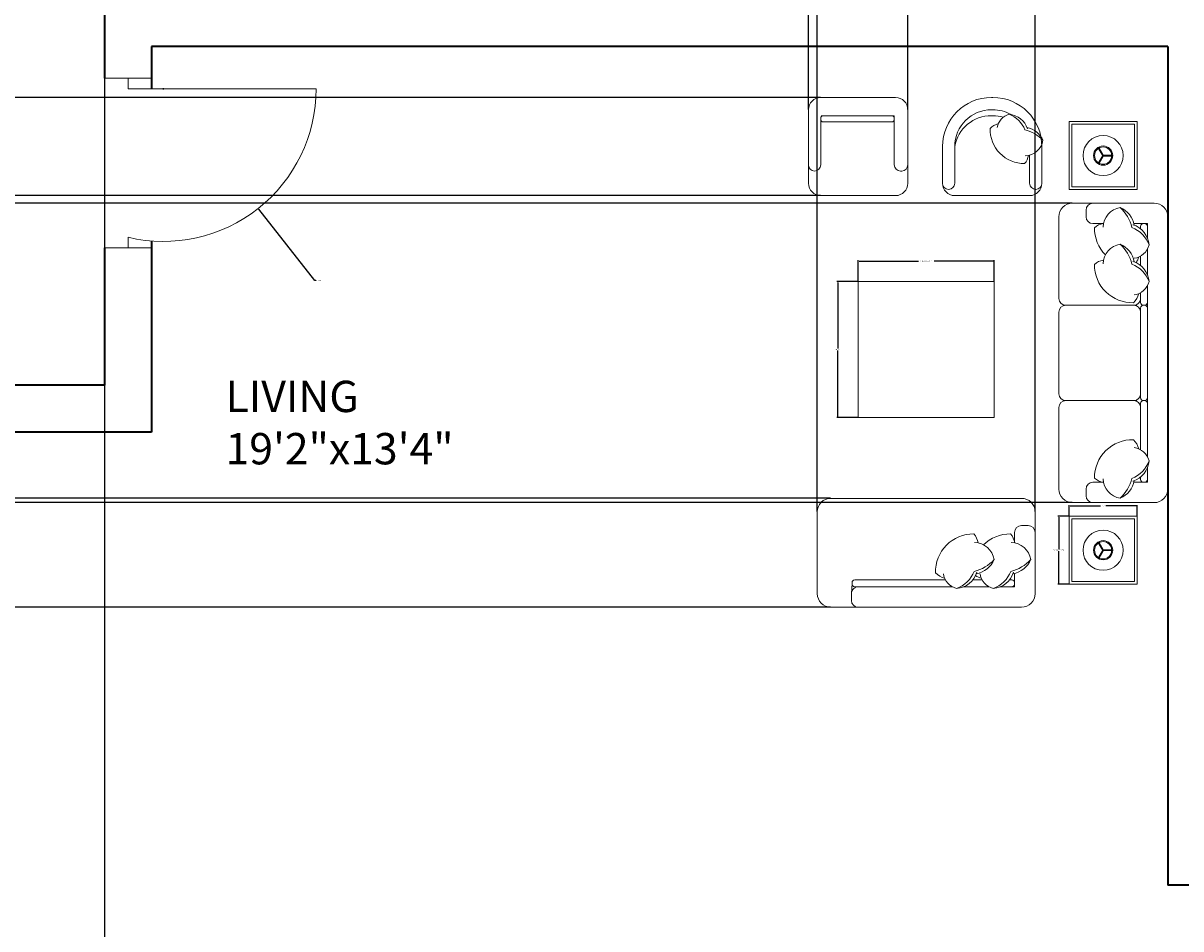
# Model space of a CAD drawing. Units: inches. Extents: x 1902 to 2626, y 1199 to 2408.
# Tile 4 of 9: x 2113 to 2334, y 1644 to 1817. Entities that reach past the tile are written whole.
import ezdxf

# ---------------------------------------------------------------- set-up
doc = ezdxf.new("R2010")
doc.units = ezdxf.units.IN
for name, color, linetype, lineweight in [('A-ANNO-DIMS', 2, 'Continuous', 18), ('A-AREA-IDEN', 7, 'Continuous', 18), ('A-DOOR', 31, 'Continuous', 18), ('A-FURN', 8, 'Continuous', 13), ('A-WALL', 7, 'Continuous', 35)]:
    doc.layers.add(name, color=color, linetype=linetype, lineweight=lineweight)
doc.styles.get("Standard").update_dxf_attribs({"font": 'arial.ttf'})
doc.dimstyles.get("Standard").update_dxf_attribs({"dimtxt": 0.18, "dimasz": 0.18, "dimexe": 0.18, "dimexo": 0.0625, "dimgap": 0.09, "dimtad": 0, "dimtih": 1, "dimtoh": 1, "dimdec": 4, "dimzin": 0, "dimdsep": 46, "dimtxsty": 'Standard', "dimcen": 0.09, "dimadec": 0, "dimazin": 0, "dimtfac": 1, "dimtdec": 4, "dimtofl": 0, "dimtmove": 0, "dimatfit": 3, "dimfxl": 1, "dimtolj": 1, "dimtzin": 0, "dimarcsym": 0})

# ---------------------------------------------------------------- blocks, each defined once
blk = doc.blocks.new('TABLE-END-WITH-LAMP')
for p, q in [((6.45, 6.47), (5.53, 8.06)), ((6.59, 6.55), (5.67, 8.14)), ((6.45, 6.55), (5.53, 4.96)), ((6.59, 6.47), (5.67, 4.88)), ((6.52, 6.59), (8.35, 6.59)), ((6.52, 6.43), (8.35, 6.43))]:
    blk.add_line(p, q)
at = {"ltscale": 0.03}
blk.add_lwpolyline([(0.01, 0), (0.01, 13.02), (13.03, 13.02), (13.03, 0)], close=True, dxfattribs=at)
blk.add_lwpolyline([(0.53, 12.5), (0.53, 0.52), (12.51, 0.52), (12.51, 12.5)], close=True)
for radius in [3.84, 1.84, 1.65]:
    blk.add_circle((6.52, 6.51), radius)
blk = doc.blocks.new('TABLE-COFFEE-SQUARE')
at = {"ltscale": 0.03}
blk.add_lwpolyline([(0, 26.05), (0, 0), (26.05, 0), (26.05, 26.05)], close=True, dxfattribs=at)
blk = doc.blocks.new('*D24')
at = {"layer": 'A-ANNO-DIMS', "color": 0, "lineweight": -2, "transparency": 16777216}
for p, q in [((2312.9, 1722.59), (2310.83, 1722.59)), ((2311.01, 1722.41), (2311.01, 1716.26)), ((2311.01, 1709.75), (2311.01, 1715.9)), ((2312.9, 1709.57), (2310.83, 1709.57))]:
    blk.add_line(p, q, dxfattribs=at)
at = {"layer": 'A-ANNO-DIMS', "color": 0, "transparency": 16777216}
for points in [[(2310.98, 1722.41), (2311.04, 1722.41), (2311.01, 1722.59)], [(2310.98, 1709.75), (2311.04, 1709.75), (2311.01, 1709.57)]]:
    blk.add_solid(points, dxfattribs=at)
at = {"layer": 'Defpoints', "color": 0, "transparency": 16777216}
for p in [(2311.01, 1722.59), (2312.97, 1722.59), (2312.97, 1709.57)]:
    blk.add_point(p, dxfattribs=at)
at = {"layer": 'A-ANNO-DIMS', "color": 0, "transparency": 16777216, "insert": (2311.01, 1716.08), "char_height": 0.18, "attachment_point": 5}
blk.add_mtext('\\A1;END TABLE 13 TYP.', dxfattribs=at)
blk = doc.blocks.new('*D25')
at = {"layer": 'A-ANNO-DIMS', "color": 0, "lineweight": -2, "transparency": 16777216}
for p, q in [((2312.97, 1722.66), (2312.97, 1724.73)), ((2313.15, 1724.55), (2318.96, 1724.55)), ((2325.81, 1724.55), (2320, 1724.55)), ((2325.99, 1722.66), (2325.99, 1724.73))]:
    blk.add_line(p, q, dxfattribs=at)
at = {"layer": 'A-ANNO-DIMS', "color": 0, "transparency": 16777216}
for points in [[(2313.15, 1724.58), (2313.15, 1724.52), (2312.97, 1724.55)], [(2325.81, 1724.58), (2325.81, 1724.52), (2325.99, 1724.55)]]:
    blk.add_solid(points, dxfattribs=at)
at = {"layer": 'Defpoints', "color": 0, "transparency": 16777216}
for p in [(2325.99, 1724.55), (2312.97, 1722.59), (2325.99, 1722.59)]:
    blk.add_point(p, dxfattribs=at)
at = {"layer": 'A-ANNO-DIMS', "color": 0, "transparency": 16777216, "insert": (2319.48, 1724.55), "char_height": 0.18, "attachment_point": 5}
blk.add_mtext('\\A1;13 TYP.', dxfattribs=at)
blk = doc.blocks.new('*D26')
at = {"layer": 'A-ANNO-DIMS', "color": 0, "lineweight": -2, "transparency": 16777216}
for p, q in [((2272.59, 1767.59), (2272.59, 1771.62)), ((2272.77, 1771.44), (2284.11, 1771.44)), ((2298.46, 1771.44), (2287.12, 1771.44)), ((2298.64, 1767.59), (2298.64, 1771.62))]:
    blk.add_line(p, q, dxfattribs=at)
at = {"layer": 'A-ANNO-DIMS', "color": 0, "transparency": 16777216}
for points in [[(2272.77, 1771.47), (2272.77, 1771.41), (2272.59, 1771.44)], [(2298.46, 1771.47), (2298.46, 1771.41), (2298.64, 1771.44)]]:
    blk.add_solid(points, dxfattribs=at)
at = {"layer": 'Defpoints', "color": 0, "transparency": 16777216}
for p in [(2298.64, 1771.44), (2272.59, 1767.53), (2298.64, 1767.53)]:
    blk.add_point(p, dxfattribs=at)
at = {"layer": 'A-ANNO-DIMS', "color": 0, "transparency": 16777216, "insert": (2285.61, 1771.44), "char_height": 0.18, "attachment_point": 5}
blk.add_mtext('\\A1;COFFEE TABLE 26 TYP.', dxfattribs=at)
blk = doc.blocks.new('*D27')
at = {"layer": 'A-ANNO-DIMS', "color": 0, "lineweight": -2, "transparency": 16777216}
for p, q in [((2272.53, 1767.53), (2268.5, 1767.53)), ((2268.68, 1767.35), (2268.68, 1754.69)), ((2268.68, 1741.66), (2268.68, 1754.32)), ((2272.53, 1741.48), (2268.5, 1741.48))]:
    blk.add_line(p, q, dxfattribs=at)
at = {"layer": 'A-ANNO-DIMS', "color": 0, "transparency": 16777216}
for points in [[(2268.65, 1767.35), (2268.71, 1767.35), (2268.68, 1767.53)], [(2268.65, 1741.66), (2268.71, 1741.66), (2268.68, 1741.48)]]:
    blk.add_solid(points, dxfattribs=at)
at = {"layer": 'Defpoints', "color": 0, "transparency": 16777216}
for p in [(2268.68, 1767.53), (2272.59, 1767.53), (2272.59, 1741.48)]:
    blk.add_point(p, dxfattribs=at)
at = {"layer": 'A-ANNO-DIMS', "color": 0, "transparency": 16777216, "insert": (2268.68, 1754.5), "char_height": 0.18, "attachment_point": 5}
blk.add_mtext('\\A1;26 TYP.', dxfattribs=at)
blk = doc.blocks.new('*D29')
at = {"layer": 'A-ANNO-DIMS', "color": 0, "lineweight": -2, "transparency": 16777216}
for p, q in [((2191.29, 2322.47), (1943.87, 2322.47)), ((1944.05, 2322.29), (1944.05, 1836.38)), ((1944.05, 1350.11), (1944.05, 1836.02)), ((2202.79, 1349.93), (1943.87, 1349.93))]:
    blk.add_line(p, q, dxfattribs=at)
at = {"layer": 'A-ANNO-DIMS', "color": 0, "transparency": 16777216}
for points in [[(1944.02, 2322.29), (1944.08, 2322.29), (1944.05, 2322.47)], [(1944.02, 1350.11), (1944.08, 1350.11), (1944.05, 1349.93)]]:
    blk.add_solid(points, dxfattribs=at)
at = {"layer": 'Defpoints', "color": 0, "transparency": 16777216}
for p in [(1944.05, 2322.47), (2191.35, 2322.47), (2202.85, 1349.93)]:
    blk.add_point(p, dxfattribs=at)
at = {"layer": 'A-ANNO-DIMS', "color": 0, "transparency": 16777216, "insert": (1944.05, 1836.2), "char_height": 0.18, "attachment_point": 5}
blk.add_mtext('\\A1;972.5', dxfattribs=at)
blk = doc.blocks.new('*D38')
at = {"layer": 'A-ANNO-DIMS', "color": 0, "lineweight": -2, "transparency": 16777216}
for p, q in [((2008.35, 1874.05), (2008.35, 1198.67)), ((2128.35, 1874.05), (2128.35, 1198.67)), ((2008.53, 1198.85), (2068.07, 1198.85)), ((2128.17, 1198.85), (2068.63, 1198.85))]:
    blk.add_line(p, q, dxfattribs=at)
at = {"layer": 'A-ANNO-DIMS', "color": 0, "transparency": 16777216}
for points in [[(2008.53, 1198.88), (2008.53, 1198.82), (2008.35, 1198.85)], [(2128.17, 1198.88), (2128.17, 1198.82), (2128.35, 1198.85)]]:
    blk.add_solid(points, dxfattribs=at)
at = {"layer": 'Defpoints', "color": 0, "transparency": 16777216}
for p in [(2008.35, 1874.11), (2128.35, 1874.11), (2128.35, 1198.85)]:
    blk.add_point(p, dxfattribs=at)
at = {"layer": 'A-ANNO-DIMS', "color": 0, "transparency": 16777216, "insert": (2068.35, 1198.85), "char_height": 0.18, "attachment_point": 5}
blk.add_mtext('\\A1;120', dxfattribs=at)
blk = doc.blocks.new('*D40')
at = {"layer": 'A-ANNO-DIMS', "color": 0, "lineweight": -2, "transparency": 16777216}
for p, q in [((2313.55, 1782.51), (1943.87, 1782.51)), ((1944.05, 1782.33), (1944.05, 1754.03)), ((1944.05, 1725.38), (1944.05, 1753.67)), ((2313.55, 1725.2), (1943.87, 1725.2))]:
    blk.add_line(p, q, dxfattribs=at)
at = {"layer": 'A-ANNO-DIMS', "color": 0, "transparency": 16777216}
for points in [[(1944.02, 1782.33), (1944.08, 1782.33), (1944.05, 1782.51)], [(1944.02, 1725.38), (1944.08, 1725.38), (1944.05, 1725.2)]]:
    blk.add_solid(points, dxfattribs=at)
at = {"layer": 'Defpoints', "color": 0, "transparency": 16777216}
for p in [(1944.05, 1782.51), (2313.62, 1782.51), (2313.62, 1725.2)]:
    blk.add_point(p, dxfattribs=at)
at = {"layer": 'A-ANNO-DIMS', "color": 0, "transparency": 16777216, "insert": (1944.05, 1753.85), "char_height": 0.18, "attachment_point": 5}
blk.add_mtext('\\A1;57.31', dxfattribs=at)
blk = doc.blocks.new('*D41')
at = {"layer": 'A-ANNO-DIMS', "color": 0, "lineweight": -2, "transparency": 16777216}
for p, q in [((2264.77, 1723.47), (2264.77, 2377.95)), ((2264.95, 2377.77), (2285.22, 2377.77)), ((2306.27, 2377.77), (2286.01, 2377.77)), ((2306.45, 1723.47), (2306.45, 2377.95))]:
    blk.add_line(p, q, dxfattribs=at)
at = {"layer": 'A-ANNO-DIMS', "color": 0, "transparency": 16777216}
for points in [[(2264.95, 2377.8), (2264.95, 2377.74), (2264.77, 2377.77)], [(2306.27, 2377.8), (2306.27, 2377.74), (2306.45, 2377.77)]]:
    blk.add_solid(points, dxfattribs=at)
at = {"layer": 'Defpoints', "color": 0, "transparency": 16777216}
for p in [(2306.45, 2377.77), (2264.77, 1723.41), (2306.45, 1723.41)]:
    blk.add_point(p, dxfattribs=at)
at = {"layer": 'A-ANNO-DIMS', "color": 0, "transparency": 16777216, "insert": (2285.61, 2377.77), "char_height": 0.18, "attachment_point": 5}
blk.add_mtext('\\A1;41.68', dxfattribs=at)
blk = doc.blocks.new('*D42')
at = {"layer": 'A-ANNO-DIMS', "color": 0, "lineweight": -2, "transparency": 16777216}
for p, q in [((2267.32, 1726.02), (1943.87, 1726.02)), ((1944.05, 1725.84), (1944.05, 1715.78)), ((1944.05, 1705.36), (1944.05, 1715.41)), ((2267.32, 1705.18), (1943.87, 1705.18))]:
    blk.add_line(p, q, dxfattribs=at)
at = {"layer": 'A-ANNO-DIMS', "color": 0, "transparency": 16777216}
for points in [[(1944.02, 1725.84), (1944.08, 1725.84), (1944.05, 1726.02)], [(1944.02, 1705.36), (1944.08, 1705.36), (1944.05, 1705.18)]]:
    blk.add_solid(points, dxfattribs=at)
at = {"layer": 'Defpoints', "color": 0, "transparency": 16777216}
for p in [(1944.05, 1726.02), (2267.38, 1726.02), (2267.38, 1705.18)]:
    blk.add_point(p, dxfattribs=at)
at = {"layer": 'A-ANNO-DIMS', "color": 0, "transparency": 16777216, "insert": (1944.05, 1715.6), "char_height": 0.18, "attachment_point": 5}
blk.add_mtext('\\A1;20.84', dxfattribs=at)
blk = doc.blocks.new('*D43')
at = {"layer": 'A-ANNO-DIMS', "color": 0, "lineweight": -2, "transparency": 16777216}
for p, q in [((2263.07, 1800.47), (2263.07, 2377.95)), ((2263.25, 2377.77), (2272.13, 2377.77)), ((2281.92, 2377.77), (2273.04, 2377.77)), ((2282.1, 1800.47), (2282.1, 2377.95))]:
    blk.add_line(p, q, dxfattribs=at)
at = {"layer": 'A-ANNO-DIMS', "color": 0, "transparency": 16777216}
for points in [[(2263.25, 2377.8), (2263.25, 2377.74), (2263.07, 2377.77)], [(2281.92, 2377.8), (2281.92, 2377.74), (2282.1, 2377.77)]]:
    blk.add_solid(points, dxfattribs=at)
at = {"layer": 'Defpoints', "color": 0, "transparency": 16777216}
for p in [(2282.1, 2377.77), (2263.07, 1800.41), (2282.1, 1800.41)]:
    blk.add_point(p, dxfattribs=at)
at = {"layer": 'A-ANNO-DIMS', "color": 0, "transparency": 16777216, "insert": (2272.58, 2377.77), "char_height": 0.18, "attachment_point": 5}
blk.add_mtext('\\A1;19.024', dxfattribs=at)
blk = doc.blocks.new('*D44')
at = {"layer": 'A-ANNO-DIMS', "color": 0, "lineweight": -2, "transparency": 16777216}
for p, q in [((2265.36, 1802.76), (1943.87, 1802.76)), ((1944.05, 1802.58), (1944.05, 1793.54)), ((1944.05, 1784.15), (1944.05, 1793.18)), ((2265.36, 1783.97), (1943.87, 1783.97))]:
    blk.add_line(p, q, dxfattribs=at)
at = {"layer": 'A-ANNO-DIMS', "color": 0, "transparency": 16777216}
for points in [[(1944.02, 1802.58), (1944.08, 1802.58), (1944.05, 1802.76)], [(1944.02, 1784.15), (1944.08, 1784.15), (1944.05, 1783.97)]]:
    blk.add_solid(points, dxfattribs=at)
at = {"layer": 'Defpoints', "color": 0, "transparency": 16777216}
for p in [(1944.05, 1802.76), (2265.42, 1802.76), (2265.42, 1783.97)]:
    blk.add_point(p, dxfattribs=at)
at = {"layer": 'A-ANNO-DIMS', "color": 0, "transparency": 16777216, "insert": (1944.05, 1793.36), "char_height": 0.18, "attachment_point": 5}
blk.add_mtext('\\A1;18.79', dxfattribs=at)
blk = doc.blocks.new('*D49')
at = {"layer": 'A-ANNO-DIMS', "color": 0, "lineweight": -2, "transparency": 16777216}
for p, q in [((2139.53, 1804.41), (2139.71, 1804.41)), ((2139.62, 1804.32), (2139.62, 1804.5)), ((2168.61, 1767.72), (2157.85, 1781.34)), ((2168.79, 1767.72), (2168.61, 1767.72))]:
    blk.add_line(p, q, dxfattribs=at)
at = {"layer": 'A-ANNO-DIMS', "color": 0, "transparency": 16777216}
blk.add_solid([(2157.87, 1781.35), (2157.83, 1781.32), (2157.74, 1781.48)], dxfattribs=at)
at = {"layer": 'Defpoints', "color": 0, "transparency": 16777216}
for p in [(2139.62, 1804.41), (2157.74, 1781.48)]:
    blk.add_point(p, dxfattribs=at)
at = {"layer": 'A-ANNO-DIMS', "color": 0, "transparency": 16777216, "insert": (2169.34, 1767.72), "char_height": 0.18, "attachment_point": 5}
blk.add_mtext('\\A1;R29.226', dxfattribs=at)

msp = doc.modelspace()

# ---------------------------------------------------------------- linework, layer by layer
at = {"layer": 'A-DOOR'}
for p, q in [((2128.3507, 1806.4133), (2137.3507, 1806.4133)), ((2137.3507, 1806.4133), (2132.8507, 1806.4133)), ((2132.8507, 1806.4133), (2132.8507, 1804.4133)), ((2132.8507, 1804.4133), (2168.8507, 1804.4133)), ((2132.8507, 1773.9835), (2132.8507, 1775.9835)), ((2128.3507, 1773.9835), (2137.3507, 1773.9835)), ((2137.3507, 1773.9835), (2132.8507, 1773.9835))]:
    msp.add_line(p, q, dxfattribs=at)
msp.add_arc((2139.6249, 1804.4133), 29.2258, 256.597574, 360, dxfattribs=at)
at = {"layer": 'A-FURN'}
msp.add_line((2271.2864, 1707.782), (2271.4129, 1709.7357), dxfattribs=at)
at = {"layer": 'A-FURN', "ltscale": 0.03}
for points in [[(2265.4197, 1802.7563), (2265.4197, 1802.7563, 0.41421356), (2263.071, 1800.4076), (2263.071, 1786.3154, 0.41421356), (2265.4197, 1783.9667), (2265.4197, 1783.9667), (2279.7467, 1783.9667, 0.41421356), (2282.0954, 1786.3154), (2282.0954, 1800.4076, 0.41421356), (2279.7467, 1802.7563)], [(2313.6163, 1725.1982, -0.41421356), (2311.0114, 1727.8031), (2311.0114, 1743.4326, -0.41421356), (2312.3138, 1744.7351, -0.41421356), (2311.0114, 1746.0375), (2311.0114, 1761.667, -0.41421356), (2312.3138, 1762.9695, -0.41421356), (2311.0114, 1764.2719), (2311.0114, 1779.9014, -0.41421356), (2313.6163, 1782.5063), (2329.2458, 1782.5063, -0.41421356), (2331.8507, 1779.9014), (2331.8507, 1727.8031, -0.41421356), (2329.2458, 1725.1982)], [(2264.7741, 1723.4115, -0.41421356), (2267.379, 1726.0164), (2267.379, 1726.0164, 0.31783725), (2267.379, 1726.0164, -0.41421356), (2267.379, 1726.0164), (2267.379, 1726.0164, 1.18618475), (2267.379, 1726.0164, -0.41421356), (2267.379, 1726.0164), (2303.8478, 1726.0164, -0.41421356), (2306.4528, 1723.4115), (2306.4528, 1707.782, -0.41421356), (2303.8478, 1705.1771), (2267.379, 1705.1771, -0.41421356), (2264.7741, 1707.782)]]:
    msp.add_lwpolyline(points, format="xyb", close=True, dxfattribs=at)
msp.add_lwpolyline([(2298.2473, 1783.9667), (2291.0838, 1783.9667, -0.41421356), (2288.7351, 1786.3154), (2288.7351, 1793.3615, -0.41421356), (2298.1298, 1802.7563), (2298.2473, 1802.7563), (2298.3647, 1802.7563, -0.41421356), (2307.7595, 1793.3615), (2307.7595, 1786.3154, -0.41421356), (2305.4108, 1783.9667), (2298.2473, 1783.9667)], format="xyb", dxfattribs=at)
at = {"layer": 'A-FURN'}
for points in [[(2291.0838, 1793.3615, -0.41421356), (2298.1298, 1800.4076), (2298.2473, 1800.4076)], [(2301.8623, 1799.4782, 0.13059149), (2298.3647, 1800.4076), (2298.2473, 1800.4076)], [(2304.9935, 1796.726, 0.30666349), (2301.4908, 1799.5253, 0.30632997), (2299.2026, 1796.9688, -0.87284716)], [(2307.9516, 1794.547, 0.14772988), (2304.5193, 1796.5652, 0.21334276), (2301.4908, 1799.5253, 0.17866181)], [(2265.4197, 1798.5286), (2265.4197, 1789.8385, -0.41421356), (2264.2453, 1788.6641), (2264.2453, 1788.6641, -0.41421356), (2263.071, 1789.8385)], [(2275.0876, 1799.2332), (2265.8894, 1799.2332, 0.41421356), (2265.4197, 1798.7635), (2265.4197, 1798.5286, 0.41421356), (2265.8894, 1798.0589), (2273.9051, 1798.0589, 0.41421356)], [(2273.9051, 1798.0589), (2279.0421, 1798.0589, 0.41421356), (2279.5118, 1798.5286), (2279.5118, 1798.7635, 0.41421356), (2279.0421, 1799.2332)], [(2279.0421, 1799.2332), (2275.0876, 1799.2332, 0.41421356)], [(2291.0838, 1793.3615, -0.37271891), (2298.1298, 1799.2332), (2298.2473, 1799.2332)], [(2305.1785, 1791.6585, -0.16554063), (2304.452, 1790.1068, -0.42598917), (2297.8566, 1796.8343, -0.12152332), (2299.4222, 1797.7615, 7.11546429)], [(2300.3669, 1798.9802, 0.07238424), (2298.3647, 1799.2332), (2298.2473, 1799.2332)], [(2304.5866, 1791.5869, 0.35677236), (2307.9516, 1794.547, 0.24954205), (2304.9026, 1796.9863, -9.61688035)], [(2291.0838, 1793.3616), (2291.0838, 1786.3154, -0.41421356), (2289.9094, 1785.1411), (2289.9094, 1785.1411, -0.41421356), (2288.7351, 1786.3154)], [(2282.0954, 1789.8385, -0.41421356), (2280.921, 1788.6641), (2280.6862, 1788.6641, -0.41421356), (2279.5118, 1789.8385), (2279.5118, 1791.6579)], [(2305.4108, 1791.715), (2305.4108, 1786.3154, 0.41421356), (2306.5851, 1785.1411), (2306.5851, 1785.1411, 0.41421356), (2307.7595, 1786.3154)], [(2319.5416, 1778.5989), (2317.5236, 1778.5989, -0.41421356), (2316.2212, 1779.9014), (2316.2212, 1781.2039, -0.41421356), (2317.5236, 1782.5063)], [(2319.4628, 1777.9453, -0.35677236), (2322.7458, 1781.6774, -0.24954205), (2325.4513, 1778.2958)], [(2322.7458, 1781.6774, -0.14772988), (2324.9842, 1777.8707, -0.21334276), (2328.2672, 1774.5118)], [(2319.5422, 1778.6018, 0.16554063), (2317.8213, 1777.796, 0.20023115), (2319.9172, 1772.6258)], [(2325.1626, 1778.3966, -0.30666349), (2328.2672, 1774.5118, -0.30632997), (2325.4319, 1771.974)], [(2327.9433, 1775.8589), (2327.9433, 1778.5989), (2325.3837, 1778.5989, -0.41435211)], [(2326.6408, 1777.605), (2326.6408, 1778.078, -0.41421356), (2327.1618, 1778.5989), (2327.4223, 1778.5989, -0.41421356), (2327.9433, 1778.078)], [(2327.9433, 1778.078), (2327.9433, 1775.8589, -0.41446868)], [(2319.4628, 1770.929, -0.35677236), (2322.7458, 1774.6611, -0.24954205), (2325.4513, 1771.2795)], [(2322.7458, 1774.6611, -0.14772988), (2324.9842, 1770.8544, -0.21334276), (2328.2672, 1767.4955)], [(2327.9433, 1773.6921), (2327.9433, 1768.8426, -0.41474665)], [(2319.5422, 1771.5855, 0.16554063), (2317.8213, 1770.7798, 0.42598917), (2325.2827, 1763.4649, 0.12152332), (2326.3111, 1765.2013)], [(2325.1626, 1771.3803, -0.30666349), (2328.2672, 1767.4955, -0.30632997), (2325.4319, 1764.9577)], [(2325.8019, 1771.1256, 0.07186538), (2326.3111, 1772.2176)], [(2326.6408, 1770.5887), (2326.6408, 1772.3806, -0.41459885)], [(2327.9433, 1766.6758), (2327.9433, 1763.4904, -0.41421356), (2327.4223, 1762.9695), (2327.1618, 1762.9695, -0.41421356), (2326.6408, 1763.4904), (2326.6408, 1765.3643, -0.12631336)], [(2326.6408, 1764.2719, -0.41421356), (2325.3384, 1762.9695), (2312.3138, 1762.9695, -0.41732018)], [(2326.6408, 1761.667, 0.41421356), (2325.3384, 1762.9695)], [(2326.6408, 1743.4326, 0.41421356), (2325.3384, 1744.7351), (2312.3138, 1744.7351, 0.4152491)], [(2326.6408, 1746.0375, -0.41421356), (2325.3384, 1744.7351)], [(2327.9433, 1734.0124), (2327.9433, 1744.2141, 0.41421356), (2327.4223, 1744.7351), (2327.1618, 1744.7351, 0.41421356), (2326.6408, 1744.2141), (2326.6408, 1735.3239, 0.41265155)], [(2319.5422, 1729.1027, -0.16554063), (2317.8213, 1729.9085, -0.42598917), (2325.2827, 1737.2233, -0.12152332), (2326.3111, 1735.4869)], [(2325.1626, 1729.3079, 0.30666349), (2328.2672, 1733.1927, 0.30632997), (2325.4319, 1735.7305)], [(2322.7458, 1726.0271, 0.14772988), (2324.9842, 1729.8338, 0.21334276), (2328.2672, 1733.1927)], [(2327.9433, 1729.6265), (2327.9433, 1731.8456, 0.41253535)], [(2317.5236, 1725.1982, -0.41421356), (2316.2212, 1726.5006), (2316.2212, 1727.8031, -0.41421356), (2317.5236, 1729.1056), (2319.5416, 1729.1056)], [(2319.4628, 1729.7592, 0.35677236), (2322.7458, 1726.0271, 0.24954205), (2325.4513, 1729.4087)], [(2326.6408, 1730.0995), (2326.6408, 1729.6265, 0.41421356), (2327.1618, 1729.1056), (2327.4223, 1729.1056, 0.41421356), (2327.9433, 1729.6265)], [(2302.5454, 1717.4861), (2302.5454, 1719.5041, -0.41421356), (2303.8478, 1720.8066), (2305.1503, 1720.8066, -0.41421356), (2306.4528, 1719.5041)], [(2295.5319, 1717.4855, 0.16554063), (2294.7262, 1719.2064, 0.42598917), (2287.4113, 1711.7451, 0.12152332), (2289.1477, 1710.7167, -7.11546429)], [(2294.8755, 1717.5649, -0.35677236), (2298.6075, 1714.2819, -0.24954205), (2295.2259, 1711.5765, 9.61688035)], [(2302.5482, 1717.4855, 0.16554063), (2301.7425, 1719.2064, 0.20023115), (2296.5722, 1717.1105, 0.12152332)], [(2301.8918, 1717.5649, -0.35677236), (2305.6238, 1714.2819, -0.24954205), (2302.2422, 1711.5765, 9.61688035)], [(2298.6075, 1714.2819, -0.14772988), (2294.8008, 1712.0435, -0.21334276), (2291.442, 1708.7605, -0.17866181)], [(2305.6238, 1714.2819, -0.14772988), (2301.8171, 1712.0435, -0.21334276), (2298.4583, 1708.7605, -0.17866181)], [(2295.3267, 1711.8651, -0.30666349), (2291.442, 1708.7605, -0.30632997), (2288.9042, 1711.5959, 0.87284716)], [(2295.0721, 1711.2259, 0.07186538), (2296.164, 1710.7167, -7.11546429)], [(2302.343, 1711.8651, -0.30666349), (2298.4583, 1708.7605, -0.30632997), (2295.9204, 1711.5959, 0.87284716)], [(2299.8054, 1709.0844), (2302.5454, 1709.0844), (2302.5454, 1711.6441, -0.41421356)], [(2274.6068, 1709.0844), (2272.5889, 1709.0844, 0.41421356), (2271.2864, 1707.782), (2271.2864, 1706.4795, 0.41421356), (2272.5889, 1705.1771)], [(2290.6223, 1709.0844), (2271.9339, 1709.0844, -0.41421356), (2271.4129, 1709.6054), (2271.4129, 1709.8659, -0.41421356), (2271.9339, 1710.3869), (2289.3108, 1710.3869, -0.41421356)], [(2297.6386, 1709.0844), (2292.7891, 1709.0844, -0.41421356)], [(2294.5352, 1710.3869), (2296.3271, 1710.3869, -0.41421356)], [(2302.0244, 1709.0844), (2299.8054, 1709.0844, -0.41421356)], [(2301.5515, 1710.3869), (2302.0244, 1710.3869, -0.41421356), (2302.5454, 1709.8659), (2302.5454, 1709.6054, -0.41421356), (2302.0244, 1709.0844)]]:
    msp.add_lwpolyline(points, format="xyb", dxfattribs=at)
for points in [[(2275.0876, 1799.2332), (2265.5371, 1799.2332)], [(2279.5118, 1791.6579), (2279.5118, 1799.2332), (2275.0876, 1799.2332)], [(2327.9433, 1768.8426), (2327.9433, 1773.6921)], [(2327.9433, 1734.0124), (2327.9433, 1766.6758)], [(2325.3837, 1729.1056), (2327.9433, 1729.1056), (2327.9433, 1731.8456)], [(2274.6068, 1709.0844), (2290.6223, 1709.0844)], [(2292.7891, 1709.0844), (2297.6386, 1709.0844)]]:
    msp.add_lwpolyline(points, dxfattribs=at)
msp.add_lwpolyline([(2327.9433, 1762.4485), (2327.9433, 1745.256, -0.41421356), (2327.4223, 1744.7351), (2327.1618, 1744.7351, -0.41421356), (2326.6408, 1745.256), (2326.6408, 1762.4485, -0.41421356), (2327.1618, 1762.9695), (2327.4223, 1762.9695, -0.41421356)], format="xyb", close=True, dxfattribs=at)
at = {"layer": 'A-WALL'}
for p, q in [((2128.3507, 1827.6338), (2128.3507, 1806.4133)), ((2128.3507, 1824.8108), (2128.3507, 1806.4133)), ((2331.8507, 1812.4733), (2137.3507, 1812.4733)), ((2137.3507, 1812.4733), (2137.3507, 1804.4133)), ((2331.8507, 1812.4733), (2331.8507, 1651.9733)), ((2137.3507, 1775.2762), (2137.3507, 1738.7028)), ((2128.3507, 1773.9835), (2128.3507, 1747.7028)), ((2128.3507, 1773.9835), (2128.3507, 1747.7028)), ((2128.3507, 1747.7028), (2091.6431, 1747.7028)), ((2137.3507, 1738.7028), (2089.3507, 1738.7028)), ((2339.0862, 1651.9733), (2331.8507, 1651.9733))]:
    msp.add_line(p, q, dxfattribs=at)

# ---------------------------------------------------------------- block references
at = {"layer": 'A-FURN'}
for name, p in [('TABLE-END-WITH-LAMP', (2312.96, 1785.1125)), ('TABLE-COFFEE-SQUARE', (2272.59, 1741.48)), ('TABLE-END-WITH-LAMP', (2312.96, 1709.57))]:
    msp.add_blockref(name, p, dxfattribs=at)

# ---------------------------------------------------------------- texts
at = {"layer": 'A-AREA-IDEN', "insert": (2151.5018, 1748.5217), "char_height": 6, "attachment_point": 1}
msp.add_mtext_dynamic_manual_height_columns('LIVING\\P19\'2"x13\'4"', width=163.729095, gutter_width=12.5, heights=[0], dxfattribs=at)

# ---------------------------------------------------------------- dimensions: what is measured, and where the dimension line sits
at = {"layer": 'A-ANNO-DIMS'}
for base, p1, p2, override, picture, middle in [((2282.0954, 2377.7733), (2263.071, 1800.4076), (2282.0954, 1800.4076), {"dimdec": 3, "dimlfac": 1, "dimrnd": 0, "dimzin": 0, "dimdsep": 46, "dimlunit": 2}, '*D43', (2272.5832, 2377.7733)), ((2306.4528, 2377.7733), (2264.7741, 1723.4115), (2306.4528, 1723.4115), {"dimdec": 2, "dimlfac": 1, "dimrnd": 0, "dimzin": 0, "dimdsep": 46, "dimlunit": 2}, '*D41', (2285.6134, 2377.7733)), ((2128.3507, 1198.8475), (2008.3507, 1874.11), (2128.3507, 1874.11), {"dimdec": 0, "dimlfac": 1, "dimrnd": 0, "dimzin": 0, "dimdsep": 46, "dimlunit": 2}, '*D38', (2068.3507, 1198.8475))]:
    dim = msp.add_linear_dim(base=base, p1=p1, p2=p2, dimstyle='Standard', override=override, dxfattribs=at)
    dim.commit()
    dim.dimension.update_dxf_attribs({"geometry": picture, "text_midpoint": middle})
for base, p1, p2, override, picture, middle in [((1944.0507, 2322.4733), (2202.8507, 1349.9322), (2191.3507, 2322.4733), {"dimdec": 1, "dimlfac": 1, "dimrnd": 0, "dimzin": 0, "dimdsep": 46, "dimlunit": 2}, '*D29', (1944.0507, 1836.2028)), ((1944.0507, 1802.7563), (2265.4197, 1783.9667), (2265.4197, 1802.7563), {"dimdec": 2, "dimlfac": 1, "dimrnd": 0, "dimzin": 0, "dimdsep": 46, "dimlunit": 2}, '*D44', (1944.0507, 1793.3615)), ((1944.0507, 1782.5063), (2313.6163, 1725.1982), (2313.6163, 1782.5063), {"dimdec": 2, "dimlfac": 1, "dimrnd": 0, "dimzin": 0, "dimdsep": 46, "dimlunit": 2}, '*D40', (1944.0507, 1753.8523)), ((1944.0507, 1726.0164), (2267.379, 1705.1771), (2267.379, 1726.0164), {"dimdec": 2, "dimlfac": 1, "dimrnd": 0, "dimzin": 0, "dimdsep": 46, "dimlunit": 2}, '*D42', (1944.0507, 1715.5967))]:
    dim = msp.add_linear_dim(base=base, p1=p1, p2=p2, angle=90, dimstyle='Standard', override=override, dxfattribs=at)
    dim.commit()
    dim.dimension.update_dxf_attribs({"geometry": picture, "text_midpoint": middle})
dim = msp.add_radius_dim(center=(2139.6249, 1804.4133), mpoint=(2157.7379, 1781.4772), dimstyle='Standard', override={"dimdec": 3, "dimlfac": 1, "dimrnd": 0, "dimzin": 0, "dimdsep": 46, "dimlunit": 2}, dxfattribs=at)
dim.commit()
dim.dimension.update_dxf_attribs({"geometry": '*D49', "text_midpoint": (2169.3353, 1767.7155), "dimtype": 164})
for base, p1, p2, text, picture, middle in [((2298.638, 1771.4354), (2272.5889, 1767.5281), (2298.638, 1767.5281), 'COFFEE TABLE <> TYP.', '*D26', (2285.6134, 1771.4354)), ((2325.9896, 1724.547), (2312.965, 1722.5933), (2325.9896, 1722.5933), '<> TYP.', '*D25', (2319.4773, 1724.547))]:
    dim = msp.add_linear_dim(base=base, p1=p1, p2=p2, text=text, dimstyle='Standard', override={"dimdec": 0, "dimlfac": 1, "dimrnd": 0, "dimzin": 0, "dimdsep": 46, "dimlunit": 2}, dxfattribs=at)
    dim.commit()
    dim.dimension.update_dxf_attribs({"geometry": picture, "text_midpoint": middle})
for base, p1, p2, text, picture, middle in [((2268.6815, 1767.5281), (2272.5889, 1741.4789), (2272.5889, 1767.5281), '<> TYP.', '*D27', (2268.6815, 1754.5035)), ((2311.0114, 1722.5933), (2312.965, 1709.5687), (2312.965, 1722.5933), 'END TABLE <> TYP.', '*D24', (2311.0114, 1716.081))]:
    dim = msp.add_linear_dim(base=base, p1=p1, p2=p2, angle=90, text=text, dimstyle='Standard', override={"dimdec": 0, "dimlfac": 1, "dimrnd": 0, "dimzin": 0, "dimdsep": 46, "dimlunit": 2}, dxfattribs=at)
    dim.commit()
    dim.dimension.update_dxf_attribs({"geometry": picture, "text_midpoint": middle})

doc.saveas('drawing.dxf')
